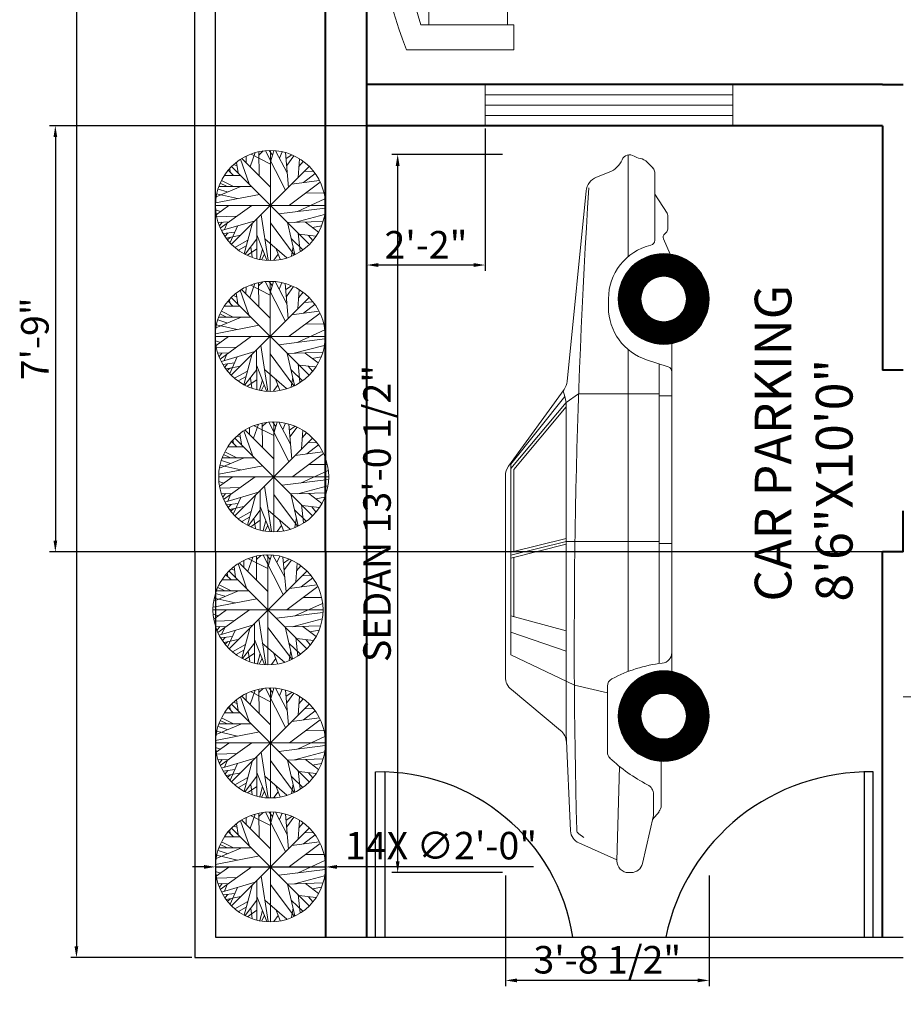
# Model space of a CAD drawing. Units: inches. Extents: x 459864 to 460310, y 324185 to 324787.
# Tile 1 of 112: x 459868 to 460061, y 324185 to 324400. Entities that reach past the tile are written whole.
import ezdxf

# ---------------------------------------------------------------- set-up
doc = ezdxf.new("R2010")
doc.units = ezdxf.units.IN
for name, color, linetype, lineweight in [('A-ANNO-DIMS', 2, 'Continuous', 18), ('A-AREA-IDEN', 7, 'Continuous', 25), ('A-FURN', 8, 'Continuous', 18), ('A-GLAZ', 4, 'Continuous', 18), ('A-WALL', 7, 'Continuous', 40), ('C-PRKG-VEHI', 8, 'Continuous', 18), ('C-PROP', 7, 'Continuous', 30), ('L-GATE', 3, 'Continuous', 25), ('L-HRDS', 9, 'Continuous', 18), ('L-PLNT', 3, 'Continuous', 13)]:
    doc.layers.add(name, color=color, linetype=linetype, lineweight=lineweight)
doc.styles.get("Standard").update_dxf_attribs({"font": 'arial.ttf'})
doc.dimstyles.new('ISO-25', dxfattribs={"dimtxt": 6, "dimasz": 2.5, "dimexe": 1.25, "dimexo": 0.625, "dimtad": 1, "dimdec": 1, "dimlunit": 3, "dimtxsty": 'Standard', "dimcen": 2.5, "dimadec": 0, "dimazin": 0, "dimtfac": 1, "dimtdec": 1, "dimtmove": 0, "dimatfit": 3, "dimfxl": 1, "dimarcsym": 0})

# ---------------------------------------------------------------- blocks, each defined once
blk = doc.blocks.new('Window - Wood Frame 36 in. Wide plan')
for p, q in [((0, 6), (0, 0)), ((36, 6), (36, 0)), ((0, 4.5), (36, 4.5)), ((0, 3), (36, 3)), ((0, 1.5), (36, 1.5))]:
    blk.add_line(p, q)
blk = doc.blocks.new('Sofa - Roundback 7 ft.')
for p, q in [((-12.00002, -32.4421), (-12.00003, -6.5971)), ((11.99997, -32.4421), (11.99998, -6.5971)), ((-36.000027, -34), (-36.000027, -11.4696)), ((35.99998, -34), (35.99998, -11.4696)), ((-35.999844, -13.3819), (35.9998, -13.3819)), ((-36.000027, -32.4421), (35.99998, -32.4421))]:
    blk.add_line(p, q)
for points in [[(-36.000027, -34), (-42.000027, -34), (-42.000027, -8)], [(41.99998, -8), (41.99998, -34), (35.99998, -34)]]:
    blk.add_lwpolyline(points)
for centre, radius, start, end in [((0, -114.25), 114.25, 68.43141, 111.5686), ((-0.00001, -127.1968), 121.1968, 72.72033, 107.2797)]:
    blk.add_arc(centre, radius, start, end)
blk = doc.blocks.new('Tree - deciduous plan')
for p, q in [((-26.4472, 46.5894), (-26.2712, 53.8116)), ((-22.0458, 42.0753), (-16.5881, 57.6486)), ((-21.1656, 55.8436), (-0.0388, 45.0094)), ((-12.5388, 54.9406), (-7.9613, 59.4546)), ((-12.3627, 32.1443), (-12.5388, 58.7776)), ((-5.3205, 59.6806), (16.5105, 16.7963)), ((2.426, 54.9406), (-1.4472, 59.9056)), ((0, 59.9996), (0, -60)), ((0.4894, 48.6208), (3.6584, 59.6806)), ((18.2711, 35.5298), (5.419, 59.6806)), ((9.8203, 51.5549), (12.8133, 58.5516)), ((19.6795, 19.5047), (16.3344, 57.6486)), ((17.0387, 51.1035), (23.2006, 55.1666)), ((17.7429, 43.6552), (25.4894, 54.2636)), ((-40.1797, 44.558), (-36.4825, 43.2038)), ((-37.0107, 47.0408), (-35.25, 35.5298)), ((-32.6092, 50.4264), (-23.2782, 23.5674)), ((-31.2008, 51.1035), (-0.2149, 20.1818)), ((31.6513, 50.8778), (30.2429, 30.5643)), ((31.1232, 42.5267), (35.8767, 48.1693)), ((-49.8627, 32.8214), (-32.7853, 32.8214)), ((-45.8134, 38.2383), (-40.5318, 33.0471)), ((-43.8768, 36.4326), (-44.405, 40.2696)), ((42, 42), (-42, -42)), ((42, -42), (-42, 42)), ((36.2288, 25.1474), (48.9049, 35.0784)), ((37.1091, 37.1098), (46.6161, 37.5612)), ((-54.7923, 24.4702), (-47.75, 21.0847)), ((-53.2078, 27.4044), (-40.1797, 20.859)), ((54.3626, 25.3731), (20.9119, 0.3198)), ((23.3767, 23.3417), (53.3063, 27.4044)), ((-59.7219, 2.8025), (-12.0106, 12.0565)), ((-32.2571, 20.6333), (-59.1937, 9.348)), ((-58.6656, 12.7336), (-35.9543, 7.5424)), ((-57.081, 17.9248), (-47.0458, 14.7649)), ((-56.0247, 20.859), (-20.8134, 20.859)), ((38.5175, 13.4107), (58.2359, 13.6364)), ((-54.6162, -24.7335), (-20.2853, 0.0941)), ((29.3626, -6.6771), (59.4682, 7.091)), ((-60, 0), (60, 0)), ((-59.7219, -4.8714), (-54.2641, -6.6771)), ((-45.2853, -0.1316), (-59.0177, -10.0627)), ((-10.074, -10.0627), (-2.5036, -59.7178)), ((9.2922, -9.1598), (59.6443, -2.8401)), ((26.3697, -18.4138), (58.9401, -9.8369)), ((-58.4895, -12.3197), (-36.4825, -11.6426)), ((-57.081, -18.4138), (-45.2853, -17.9624)), ((-52.6797, -18.188), (-55.4966, -22.0251)), ((-53.2078, -27.442), (-16.7641, -16.6081)), ((-47.2219, -19.3166), (-50.2148, -26.3135)), ((-19.9331, -20.2194), (-28.5599, -52.721)), ((-14.8275, -15.0282), (-14.6515, -57.6865)), ((-0.0388, -19.0909), (25.8415, -53.8495)), ((18.6232, -18.6394), (26.7218, -53.3981)), ((18.7992, -18.6394), (57.3556, -17.2853)), ((38.1654, -18.188), (52.426, -29.0219)), ((-38.9472, -29.0219), (-51.4472, -30.6018)), ((-46.5177, -30.1504), (-49.5106, -33.536)), ((-35.9543, -22.4765), (-44.0529, -40.5329)), ((-14.6515, -32.1818), (-3.912, -59.4922)), ((30.419, -30.1504), (32.3556, -50.0125)), ((31.4753, -31.279), (49.6091, -33.3103)), ((45.9119, -24.0564), (55.595, -22.2508)), ((-32.4331, -32.4075), (-48.1021, -35.5674)), ((-43.7008, -34.6645), (-46.6937, -37.373)), ((-24.6867, -37.8244), (-38.7712, -45.7241)), ((-14.6515, -36.2445), (-27.6797, -52.9467)), ((-6.2008, -36.2445), (17.919, -57.0094)), ((22.8485, -36.4702), (35.3485, -48.4326)), ((41.5105, -32.6332), (46.088, -38.0501)), ((-26.2712, -43.9185), (-34.7219, -48.6583)), ((-14.6515, -47.3041), (-25.0388, -54.3009)), ((-21.5177, -45.4984), (-19.9331, -56.1065)), ((-8.4895, -47.5298), (-11.4825, -58.5893)), ((-6.3768, -52.721), (-9.3698, -58.815)), ((8.4119, -53.1724), (3.8344, -59.4922)), ((5.9471, -46.6269), (10.5246, -58.5893)), ((24.7852, -44.8213), (23.0246, -54.978))]:
    blk.add_line(p, q)
blk.add_circle((0, 0), 60)
blk = doc.blocks.new('Car - sedan  side')
for p, q in [((-139.53, 35.99), (-129.64, 47.91)), ((-128.57, 32.64), (-121.22, 48.02)), ((-77.81, 49.34), (-126.58, 49.34)), ((-74.7, 48.02), (-121.22, 48.02)), ((-120.32, 34.67), (-115.67, 48.02)), ((-115.4, 34.67), (-111.74, 48.02)), ((-94.41, 34.67), (-97.73, 48.02)), ((-93.72, 34.67), (-97.04, 48.02)), ((-93.03, 34.67), (-96.34, 48.02)), ((-60.02, 34.65), (-76.07, 48.02)), ((-56.87, 35.13), (-75.48, 48.59)), ((-58.54, 34.93), (-74.99, 48.02)), ((-97.55, 47.3), (-111.94, 47.3)), ((-76.26, 47.3), (-96.16, 47.3)), ((-61.08, 34.66), (-76.26, 47.3)), ((-140.23, 34.67), (-163.88, 33.56)), ((-62.28, 34.67), (-140.23, 34.67)), ((-93.72, 19.62), (-93.72, 34.67)), ((-62.28, 34.67), (-60.02, 34.65)), ((-60.02, 34.65), (-58.54, 34.93)), ((-57.97, 31.61), (-60.02, 34.65)), ((-57.21, 35.38), (-58.54, 34.93)), ((-54.93, 34.4), (-8.75, 29.8)), ((-170.93, 22.32), (-166.81, 31.56)), ((-164.57, 31.6), (-165.48, 30.35)), ((-130.39, 24.63), (-128.57, 32.64)), ((-57.97, 19.62), (-57.97, 31.61)), ((-4.21, 24.18), (-5.42, 27.27)), ((-128.78, 24.63), (-144.79, 24.63)), ((-36.97, 24.38), (-34.94, 24.38)), ((-148.26, 21.7), (-171.11, 22.33)), ((-174, 19.51), (-174, 18.91)), ((-47.2, 19.62), (-125.23, 19.62)), ((-93.72, 12.14), (-93.72, 19.62)), ((-57.97, 12.14), (-57.97, 19.62)), ((0, 19.62), (-24.7, 19.62)), ((-160.12, 13.48), (-171.81, 16.16)), ((-51.4, 9.89), (-49.69, 15.14)), ((-3.22, 13.59), (-1.77, 14.97)), ((-159.22, 12.14), (-161.08, 13.7)), ((-155.01, 13.48), (-160.12, 13.48)), ((-50.67, 12.14), (-123.32, 12.14)), ((-94.21, 9.03), (-94.21, 12.14)), ((-58.39, 9.03), (-58.39, 12.14)), ((-4.23, 13.19), (-20.72, 13.19)), ((-9.5, 13.19), (-14.1, 10.2)), ((-147.03, 11.6), (-157.73, 11.6)), ((-20.36, 11.06), (-24.06, 9.44)), ((-18.83, 10.42), (-19.11, 10.76)), ((-14.68, 10.03), (-18.01, 10.03)), ((-120.62, 9.03), (-125.23, 9.03)), ((-45.76, 9.03), (-120.62, 9.03))]:
    blk.add_line(p, q)
at = {"const_width": 5.49}
for points in [[(-127.8, 11, -1), (-144.3, 11, -1)], [(-26.69, 11, -1), (-43.19, 11, -1)]]:
    blk.add_lwpolyline(points, format="xyb", close=True, dxfattribs=at)
for centre, radius in [((-136.05, 11), 11), ((-34.94, 11), 11), ((-136.05, 11), 5.51), ((-34.94, 11), 5.51)]:
    blk.add_circle(centre, radius)
for centre, radius, start, end in [((-126.58, 45.38), 3.97, 90, 140.3029), ((-77.81, 45.38), 3.97, 54.135, 90), ((-142.58, 38.53), 3.97, 272.6827, 320.3029), ((-163.72, 30.18), 3.38, 92.6827, 155.9736), ((-54.54, 38.35), 3.97, 234.135, 264.3123), ((-163.62, 30.91), 1.17, 91.491, 143.9553), ((-118.51, -1702.12), 1734.79, 86.34698, 91.49105), ((-9.15, 25.82), 4, 21.3107, 84.3123), ((-118.09, -2.78), 38.85, 136.3964, 152.9097), ((-144.79, 22.64), 1.98, 90, 136.3964), ((-128.78, 22.64), 1.98, 28.1371, 90), ((-36.97, 11), 13.38, 90, 161.9732), ((-34.94, 11), 13.38, 13.5864, 90), ((0.9, 26.18), 5.49, 201.3107, 247.7048), ((-171.18, 19.51), 2.82, 88.4193, 180), ((-157.14, 7.48), 34.14, 6.5135, 28.1371), ((-1.92, 19.3), 1.94, 325.3744, 67.7048), ((-171.18, 18.91), 2.82, 180, 257.0905), ((-3.82, 17.12), 2.96, 313.7173, 352.3839), ((2.46, 16.28), 3.37, 145.3744, 172.3839), ((-155.01, 16.1), 2.62, 270, 332.9097), ((-157.73, 13.93), 2.32, 230.1291, 270), ((-20.72, 14.43), 1.24, 193.5864, 270), ((-4.23, 14.65), 1.46, 270, 313.7173), ((-120.62, 11.65), 2.62, 186.5135, 270), ((-52.58, 10.27), 1.24, 270, 341.9732), ((-19.93, 10.09), 1.06, 39.301, 113.7159), ((-18.01, 11.09), 1.06, 219.301, 270), ((-14.68, 11.09), 1.06, 270, 303.047)]:
    blk.add_arc(centre, radius, start, end)
blk = doc.blocks.new('*D22')
at = {"layer": 'A-ANNO-DIMS', "color": 0, "lineweight": -2, "transparency": 16777216}
for p, q in [((459905.99, 324743.98), (459879.56, 324743.98)), ((459880.81, 324741.48), (459880.81, 324197.48)), ((459905.99, 324194.98), (459879.56, 324194.98))]:
    blk.add_line(p, q, dxfattribs=at)
at = {"layer": 'A-ANNO-DIMS', "color": 0, "transparency": 16777216}
for points in [[(459880.39, 324741.48), (459881.22, 324741.48), (459880.81, 324743.98)], [(459880.39, 324197.48), (459881.22, 324197.48), (459880.81, 324194.98)]]:
    blk.add_solid(points, dxfattribs=at)
at = {"layer": 'Defpoints', "color": 0, "transparency": 16777216}
for p in [(459906.61, 324743.98), (459880.81, 324194.98), (459906.61, 324194.98)]:
    blk.add_point(p, dxfattribs=at)
at = {"layer": 'A-ANNO-DIMS', "color": 0, "transparency": 16777216, "insert": (459877.12, 324469.48), "char_height": 6, "attachment_point": 5, "rotation": 90}
blk.add_mtext('45\'-9"', dxfattribs=at)
blk = doc.blocks.new('*D46')
at = {"layer": 'A-ANNO-DIMS', "color": 0, "lineweight": -2, "transparency": 16777216}
for p, q in [((459973.74, 324370.22), (459949.61, 324370.22)), ((459950.86, 324216.02), (459950.86, 324367.72)), ((459973.74, 324213.52), (459949.61, 324213.52))]:
    blk.add_line(p, q, dxfattribs=at)
at = {"layer": 'A-ANNO-DIMS', "color": 0, "transparency": 16777216}
for points in [[(459950.44, 324367.72), (459951.27, 324367.72), (459950.86, 324370.22)], [(459950.44, 324216.02), (459951.27, 324216.02), (459950.86, 324213.52)]]:
    blk.add_solid(points, dxfattribs=at)
at = {"layer": 'Defpoints', "color": 0, "transparency": 16777216}
for p in [(459950.86, 324370.22), (459974.36, 324370.22), (459974.36, 324213.52)]:
    blk.add_point(p, dxfattribs=at)
at = {"layer": 'A-ANNO-DIMS', "color": 0, "transparency": 16777216, "insert": (459947.13, 324291.87), "char_height": 6, "attachment_point": 5, "rotation": 90}
blk.add_mtext('SEDAN 13\'-0 1/2"', dxfattribs=at)
blk = doc.blocks.new('*D47')
at = {"layer": 'A-ANNO-DIMS', "color": 0, "lineweight": -2, "transparency": 16777216}
for p, q in [((459974.36, 324212.89), (459974.36, 324188.76)), ((460018.77, 324212.89), (460018.77, 324188.76)), ((460016.27, 324190.01), (459976.86, 324190.01))]:
    blk.add_line(p, q, dxfattribs=at)
at = {"layer": 'A-ANNO-DIMS', "color": 0, "transparency": 16777216}
for points in [[(459976.86, 324190.43), (459976.86, 324189.6), (459974.36, 324190.01)], [(460016.27, 324190.43), (460016.27, 324189.6), (460018.77, 324190.01)]]:
    blk.add_solid(points, dxfattribs=at)
at = {"layer": 'Defpoints', "color": 0, "transparency": 16777216}
for p in [(459974.36, 324213.52), (460018.77, 324213.52), (459974.36, 324190.01)]:
    blk.add_point(p, dxfattribs=at)
at = {"layer": 'A-ANNO-DIMS', "color": 0, "transparency": 16777216, "insert": (459996.57, 324193.74), "char_height": 6, "attachment_point": 5}
blk.add_mtext('3\'-8 1/2"', dxfattribs=at)
blk = doc.blocks.new('*D68')
at = {"layer": 'A-ANNO-DIMS', "color": 0, "lineweight": -2, "transparency": 16777216}
for p, q in [((459944.11, 324375.86), (459944.11, 324344.83)), ((459969.94, 324375.86), (459969.94, 324344.83)), ((459967.44, 324346.08), (459946.61, 324346.08))]:
    blk.add_line(p, q, dxfattribs=at)
at = {"layer": 'A-ANNO-DIMS', "color": 0, "transparency": 16777216}
for points in [[(459946.61, 324346.5), (459946.61, 324345.67), (459944.11, 324346.08)], [(459967.44, 324346.5), (459967.44, 324345.67), (459969.94, 324346.08)]]:
    blk.add_solid(points, dxfattribs=at)
at = {"layer": 'Defpoints', "color": 0, "transparency": 16777216}
for p in [(459944.11, 324376.48), (459969.94, 324376.48), (459944.11, 324346.08)]:
    blk.add_point(p, dxfattribs=at)
at = {"layer": 'A-ANNO-DIMS', "color": 0, "transparency": 16777216, "insert": (459957.03, 324349.72), "char_height": 6, "attachment_point": 5}
blk.add_mtext('2\'-2"', dxfattribs=at)
blk = doc.blocks.new('*D69')
at = {"layer": 'A-ANNO-DIMS', "color": 0, "lineweight": -2, "transparency": 16777216}
for p, q in [((460055.99, 324376.48), (459874.96, 324376.48)), ((459876.21, 324373.98), (459876.21, 324285.98)), ((460060.49, 324283.48), (459874.96, 324283.48))]:
    blk.add_line(p, q, dxfattribs=at)
at = {"layer": 'A-ANNO-DIMS', "color": 0, "transparency": 16777216}
for points in [[(459875.8, 324373.98), (459876.63, 324373.98), (459876.21, 324376.48)], [(459875.8, 324285.98), (459876.63, 324285.98), (459876.21, 324283.48)]]:
    blk.add_solid(points, dxfattribs=at)
at = {"layer": 'Defpoints', "color": 0, "transparency": 16777216}
for p in [(460056.61, 324376.48), (459876.21, 324283.48), (460061.11, 324283.48)]:
    blk.add_point(p, dxfattribs=at)
at = {"layer": 'A-ANNO-DIMS', "color": 0, "transparency": 16777216, "insert": (459872.53, 324329.98), "char_height": 6, "attachment_point": 5, "rotation": 90}
blk.add_mtext('7\'-9"', dxfattribs=at)
blk = doc.blocks.new('*D70')
at = {"layer": 'A-ANNO-DIMS', "color": 0, "lineweight": -2, "transparency": 16777216}
for p, q in [((459908.61, 324214.77), (459906.11, 324214.77)), ((459911.11, 324214.77), (459935.11, 324214.77)), ((459980.51, 324214.78), (459937.61, 324214.77))]:
    blk.add_line(p, q, dxfattribs=at)
at = {"layer": 'A-ANNO-DIMS', "color": 0, "transparency": 16777216}
for points in [[(459908.61, 324215.19), (459908.61, 324214.36), (459911.11, 324214.77)], [(459937.61, 324215.19), (459937.61, 324214.36), (459935.11, 324214.77)]]:
    blk.add_solid(points, dxfattribs=at)
at = {"layer": 'Defpoints', "color": 0, "transparency": 16777216}
for p in [(459911.11, 324214.77), (459935.11, 324214.77)]:
    blk.add_point(p, dxfattribs=at)
at = {"layer": 'A-ANNO-DIMS', "color": 0, "transparency": 16777216, "insert": (459960.31, 324218.63), "char_height": 6, "attachment_point": 5, "rotation": 0.0017}
blk.add_mtext('14X ∅2\'-0"', dxfattribs=at)

msp = doc.modelspace()

# ---------------------------------------------------------------- linework, layer by layer
at = {"layer": 'A-WALL'}
for p, q in [((459935.11, 324283.48), (459935.11, 324715.48)), ((459944.11, 324283.48), (459944.11, 324706.48)), ((460056.61, 324385.48), (459944.11, 324385.48)), ((460056.61, 324385.48), (460060.07, 324385.48)), ((460060.07, 324385.48), (460061.11, 324385.48)), ((460056.61, 324376.48), (459944.11, 324376.48)), ((460056.61, 324376.48), (460056.61, 324323.13)), ((460061.11, 324323.13), (460056.61, 324323.13)), ((460061.11, 324283.48), (460061.11, 324292.48)), ((459935.11, 324283.48), (459935.11, 324235.48)), ((459944.11, 324199.48), (459944.11, 324283.48)), ((460056.61, 324199.48), (460056.61, 324283.48)), ((460061.11, 324283.48), (460056.61, 324283.48)), ((459935.11, 324235.48), (459935.11, 324199.48))]:
    msp.add_line(p, q, dxfattribs=at)
at = {"layer": 'C-PROP'}
for p, q in [((459906.61, 324283.48), (459906.61, 324743.98)), ((459911.11, 324283.48), (459911.11, 324739.48)), ((459906.61, 324283.48), (459906.61, 324194.98)), ((459911.11, 324283.48), (459911.11, 324199.48)), ((459911.11, 324199.48), (460061.11, 324199.48)), ((459906.61, 324194.98), (460061.11, 324194.98))]:
    msp.add_line(p, q, dxfattribs=at)
at = {"layer": 'L-GATE'}
for p, q in [((459946.05, 324235.48), (459946.11, 324235.48)), ((459946.05, 324199.48), (459946.05, 324235.48)), ((459948.05, 324235.48), (459948.05, 324199.48)), ((460052.55, 324235.48), (460052.55, 324199.48)), ((460054.55, 324199.48), (460054.55, 324235.48))]:
    msp.add_line(p, q, dxfattribs=at)
for centre, radius, start, end in [((459947.05, 324192.99), 42.5, 8.7832, 91.3482), ((460053.55, 324190.33), 45.16, 88.7312, 168.31)]:
    msp.add_arc(centre, radius, start, end, dxfattribs=at)
at = {"layer": 'L-HRDS'}
msp.add_line((460061.11, 324251.88), (460077.91, 324251.88), dxfattribs=at)

# ---------------------------------------------------------------- block references
at = {"layer": 'A-FURN', "xscale": 0.9, "yscale": 0.9, "rotation": 90}
msp.add_blockref('Sofa - Roundback 7 ft.', (459945.61, 324430.86), dxfattribs=at)
at = {"layer": 'A-GLAZ', "xscale": 1.5, "yscale": 1.5, "zscale": 1.5}
msp.add_blockref('Window - Wood Frame 36 in. Wide plan', (459969.94, 324376.48), dxfattribs=at)
at = {"layer": 'C-PRKG-VEHI', "xscale": 0.9, "yscale": 0.9, "rotation": 90}
msp.add_blockref('Car - sedan  side', (460018.77, 324370.12), dxfattribs=at)
at = {"layer": 'L-PLNT', "xscale": 0.2, "yscale": 0.2}
for p in [(459923.11, 324359.07), (459923.05, 324330.52), (459923.83, 324299.86), (459922.58, 324270.85), (459923.11, 324241.81), (459923.11, 324214.77)]:
    msp.add_blockref('Tree - deciduous plan', p, dxfattribs=at)

# ---------------------------------------------------------------- texts
at = {"layer": 'A-AREA-IDEN', "insert": (460028.72, 324272.66), "char_height": 8, "width": 253.3207, "attachment_point": 1, "rotation": 90}
msp.add_mtext('CAR PARKING\\P8\'6"X10\'0"', dxfattribs=at)

# ---------------------------------------------------------------- dimensions: what is measured, and where the dimension line sits
at = {"layer": 'A-ANNO-DIMS'}
for base, p1, p2, angle, override, picture, middle in [((459880.81, 324194.98), (459906.61, 324743.98), (459906.61, 324194.98), 90, {"dimclrd": 0, "dimclre": 0, "dimclrt": 0}, '*D22', (459877.12, 324469.48)), ((459876.21, 324283.48), (460056.61, 324376.48), (460061.11, 324283.48), 90, {"dimdec": 1, "dimlfac": 1, "dimrnd": 0, "dimzin": 1, "dimdsep": 46, "dimlunit": 4, "dimfrac": 2}, '*D69', (459872.53, 324329.98)), ((459944.11, 324346.08), (459969.94, 324376.48), (459944.11, 324376.48), 180, {"dimdec": 1, "dimlfac": 1, "dimrnd": 0, "dimzin": 1, "dimdsep": 46, "dimlunit": 4, "dimfrac": 2}, '*D68', (459957.03, 324349.72)), ((459974.36, 324190.01), (460018.77, 324213.52), (459974.36, 324213.52), 180, {"dimdec": 1, "dimlfac": 1, "dimrnd": 0, "dimzin": 1, "dimdsep": 46, "dimlunit": 4, "dimfrac": 2}, '*D47', (459996.57, 324193.74))]:
    dim = msp.add_linear_dim(base=base, p1=p1, p2=p2, angle=angle, dimstyle='ISO-25', override=override, dxfattribs=at)
    dim.commit()
    dim.dimension.update_dxf_attribs({"geometry": picture, "text_midpoint": middle})
dim = msp.add_linear_dim(base=(459950.86, 324370.22), p1=(459974.36, 324213.52), p2=(459974.36, 324370.22), angle=90, text='SEDAN <>', dimstyle='ISO-25', override={"dimdec": 1, "dimlfac": 1, "dimrnd": 0, "dimzin": 1, "dimdsep": 46, "dimlunit": 4, "dimfrac": 2}, dxfattribs=at)
dim.commit()
dim.dimension.update_dxf_attribs({"geometry": '*D46', "text_midpoint": (459947.13, 324291.87)})
dim = msp.add_diameter_dim_2p(p1=(459911.11, 324214.77), p2=(459935.11, 324214.77), text='14X <>', dimstyle='ISO-25', override={"dimdec": 1, "dimlfac": 1, "dimrnd": 0, "dimzin": 1, "dimdsep": 46, "dimlunit": 4, "dimfrac": 2}, dxfattribs=at)
dim.commit()
dim.dimension.update_dxf_attribs({"geometry": '*D70', "text_midpoint": (459960.31, 324214.77), "dimtype": 163})

doc.saveas('drawing.dxf')
